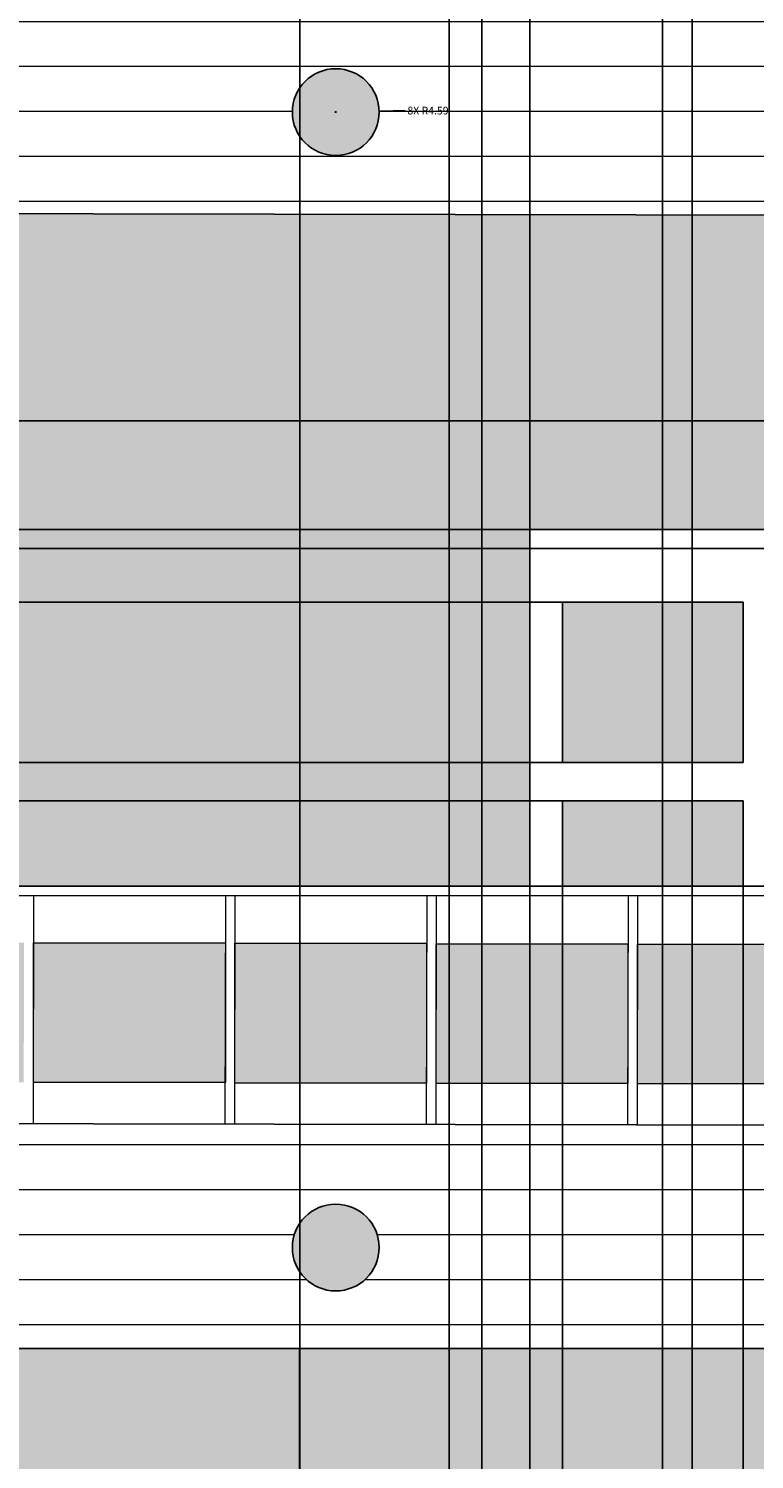
# Model space of a CAD drawing. Units: inches. Extents: x 36 to 594, y 79 to 831.
# Tile 9 of 30: x 188 to 265, y 294 to 446. Entities that reach past the tile are written whole.
import ezdxf

# ---------------------------------------------------------------- set-up
doc = ezdxf.new("R2010")
doc.units = ezdxf.units.IN
doc.header["$MEASUREMENT"] = 0
for name, color, linetype, lineweight in [('A-ANNO-DIMS', 2, 'Continuous', 18), ('A-ELEV', 7, 'Continuous', 25), ('A-ELEV-PATT', 8, 'Continuous', 13), ('A-GLAZ', 4, 'Continuous', 18)]:
    doc.layers.add(name, color=color, linetype=linetype, lineweight=lineweight)
doc.styles.get("Standard").update_dxf_attribs({"font": 'arial.ttf'})
doc.dimstyles.get("Standard").update_dxf_attribs({"dimtxt": 0.8125, "dimasz": 0.18, "dimexe": 0.18, "dimexo": 0.0625, "dimgap": 0.09, "dimtad": 0, "dimtih": 1, "dimtoh": 1, "dimdec": 4, "dimzin": 0, "dimdsep": 46, "dimlunit": 4, "dimtxsty": 'Standard', "dimcen": 0.09, "dimadec": 0, "dimazin": 0, "dimtfac": 1, "dimtdec": 4, "dimtofl": 0, "dimtmove": 0, "dimatfit": 3, "dimfxl": 1, "dimtolj": 1, "dimtzin": 0, "dimarcsym": 0})

# ---------------------------------------------------------------- blocks, each defined once
blk = doc.blocks.new('GLAZ-PANEL')
blk.add_lwpolyline([(0, 14.77), (20.28, 14.77), (20.28, 0), (0, 0)], close=True)
blk = doc.blocks.new('*D28')
at = {"layer": 'A-ANNO-DIMS', "color": 0, "lineweight": -2, "transparency": 16777216}
for p, q in [((269.3, 796.05), (37.49, 796.05)), ((37.67, 795.87), (37.67, 455.63)), ((37.67, 114.39), (37.67, 454.62)), ((94.8, 114.21), (37.49, 114.21))]:
    blk.add_line(p, q, dxfattribs=at)
at = {"layer": 'A-ANNO-DIMS', "color": 0, "transparency": 16777216}
for points in [[(37.64, 795.87), (37.7, 795.87), (37.67, 796.05)], [(37.64, 114.39), (37.7, 114.39), (37.67, 114.21)]]:
    blk.add_solid(points, dxfattribs=at)
at = {"layer": 'Defpoints', "color": 0, "transparency": 16777216}
for p in [(37.67, 796.05), (269.36, 796.05), (94.87, 114.21)]:
    blk.add_point(p, dxfattribs=at)
at = {"layer": 'A-ANNO-DIMS', "color": 0, "transparency": 16777216, "insert": (37.67, 455.13), "char_height": 0.812, "attachment_point": 5}
blk.add_mtext('\\A1;681.8', dxfattribs=at)
blk = doc.blocks.new('*D61')
at = {"layer": 'A-ANNO-DIMS', "color": 0, "lineweight": -2, "transparency": 16777216}
for p, q in [((156.41, 264.68), (156.41, 830.73)), ((156.59, 830.55), (185.26, 830.55)), ((216.85, 830.55), (188.18, 830.55)), ((217.03, 286.24), (217.03, 830.73))]:
    blk.add_line(p, q, dxfattribs=at)
at = {"layer": 'A-ANNO-DIMS', "color": 0, "transparency": 16777216}
for points in [[(156.59, 830.58), (156.59, 830.52), (156.41, 830.55)], [(216.85, 830.58), (216.85, 830.52), (217.03, 830.55)]]:
    blk.add_solid(points, dxfattribs=at)
at = {"layer": 'Defpoints', "color": 0, "transparency": 16777216}
for p in [(217.03, 830.55), (217.03, 286.18), (156.41, 264.62)]:
    blk.add_point(p, dxfattribs=at)
at = {"layer": 'A-ANNO-DIMS', "color": 0, "transparency": 16777216, "insert": (186.72, 830.55), "char_height": 0.812, "attachment_point": 5}
blk.add_mtext('\\A1;60.62', dxfattribs=at)
blk = doc.blocks.new('*D96')
at = {"layer": 'A-ANNO-DIMS', "color": 0, "lineweight": -2, "transparency": 16777216}
for p, q in [((236.29, 484.36), (236.29, 79.53)), ((232.82, 475.35), (232.82, 79.53)), ((233, 79.71), (233.41, 79.71)), ((236.11, 79.71), (235.7, 79.71))]:
    blk.add_line(p, q, dxfattribs=at)
at = {"layer": 'A-ANNO-DIMS', "color": 0, "transparency": 16777216}
for points in [[(233, 79.74), (233, 79.68), (232.82, 79.71)], [(236.11, 79.74), (236.11, 79.68), (236.29, 79.71)]]:
    blk.add_solid(points, dxfattribs=at)
at = {"layer": 'Defpoints', "color": 0, "transparency": 16777216}
for p in [(236.29, 484.42), (232.82, 475.41), (236.29, 79.71)]:
    blk.add_point(p, dxfattribs=at)
at = {"layer": 'A-ANNO-DIMS', "color": 0, "transparency": 16777216, "insert": (234.56, 79.71), "char_height": 0.812, "attachment_point": 5}
blk.add_mtext('\\A1;3.47', dxfattribs=at)
blk = doc.blocks.new('*D97')
at = {"layer": 'A-ANNO-DIMS', "color": 0, "lineweight": -2, "transparency": 16777216}
for p, q in [((236.29, 484.36), (236.29, 79.53)), ((255.36, 484.36), (255.36, 79.53)), ((236.47, 79.71), (244.09, 79.71)), ((255.18, 79.71), (247.56, 79.71))]:
    blk.add_line(p, q, dxfattribs=at)
at = {"layer": 'A-ANNO-DIMS', "color": 0, "transparency": 16777216}
for points in [[(236.47, 79.74), (236.47, 79.68), (236.29, 79.71)], [(255.18, 79.74), (255.18, 79.68), (255.36, 79.71)]]:
    blk.add_solid(points, dxfattribs=at)
at = {"layer": 'Defpoints', "color": 0, "transparency": 16777216}
for p in [(236.29, 484.42), (255.36, 484.42), (255.36, 79.71)]:
    blk.add_point(p, dxfattribs=at)
at = {"layer": 'A-ANNO-DIMS', "color": 0, "transparency": 16777216, "insert": (245.82, 79.71), "char_height": 0.812, "attachment_point": 5}
blk.add_mtext('\\A1;19.064', dxfattribs=at)
blk = doc.blocks.new('*D98')
at = {"layer": 'A-ANNO-DIMS', "color": 0, "lineweight": -2, "transparency": 16777216}
for p, q in [((255.36, 484.36), (255.36, 79.53)), ((258.51, 475.35), (258.51, 79.53)), ((255.54, 79.71), (255.78, 79.71)), ((258.33, 79.71), (258.08, 79.71))]:
    blk.add_line(p, q, dxfattribs=at)
at = {"layer": 'A-ANNO-DIMS', "color": 0, "transparency": 16777216}
for points in [[(255.54, 79.74), (255.54, 79.68), (255.36, 79.71)], [(258.33, 79.74), (258.33, 79.68), (258.51, 79.71)]]:
    blk.add_solid(points, dxfattribs=at)
at = {"layer": 'Defpoints', "color": 0, "transparency": 16777216}
for p in [(255.36, 484.42), (258.51, 475.41), (258.51, 79.71)]:
    blk.add_point(p, dxfattribs=at)
at = {"layer": 'A-ANNO-DIMS', "color": 0, "transparency": 16777216, "insert": (256.93, 79.71), "char_height": 0.812, "attachment_point": 5}
blk.add_mtext('\\A1;3.15', dxfattribs=at)
blk = doc.blocks.new('*D105')
at = {"layer": 'A-ANNO-DIMS', "color": 0, "lineweight": -2, "transparency": 16777216}
for p, q in [((241.36, 404.34), (241.36, 830.73)), ((241.54, 830.55), (252.42, 830.55)), ((266.86, 830.55), (255.98, 830.55)), ((267.04, 404.34), (267.04, 830.73))]:
    blk.add_line(p, q, dxfattribs=at)
at = {"layer": 'A-ANNO-DIMS', "color": 0, "transparency": 16777216}
for points in [[(241.54, 830.58), (241.54, 830.52), (241.36, 830.55)], [(266.86, 830.58), (266.86, 830.52), (267.04, 830.55)]]:
    blk.add_solid(points, dxfattribs=at)
at = {"layer": 'Defpoints', "color": 0, "transparency": 16777216}
for p in [(267.04, 830.55), (241.36, 404.27), (267.04, 404.27)]:
    blk.add_point(p, dxfattribs=at)
at = {"layer": 'A-ANNO-DIMS', "color": 0, "transparency": 16777216, "insert": (254.2, 830.55), "char_height": 0.812, "attachment_point": 5}
blk.add_mtext('\\A1;25.684', dxfattribs=at)
blk = doc.blocks.new('*D108')
at = {"layer": 'A-ANNO-DIMS', "color": 0, "lineweight": -2, "transparency": 16777216}
for p, q in [((244.82, 364.03), (244.82, 79.53)), ((241.36, 355.02), (241.36, 79.53)), ((241.54, 79.71), (241.95, 79.71)), ((244.64, 79.71), (244.24, 79.71))]:
    blk.add_line(p, q, dxfattribs=at)
at = {"layer": 'A-ANNO-DIMS', "color": 0, "transparency": 16777216}
for points in [[(241.54, 79.74), (241.54, 79.68), (241.36, 79.71)], [(244.64, 79.74), (244.64, 79.68), (244.82, 79.71)]]:
    blk.add_solid(points, dxfattribs=at)
at = {"layer": 'Defpoints', "color": 0, "transparency": 16777216}
for p in [(244.82, 364.09), (241.36, 355.08), (244.82, 79.71)]:
    blk.add_point(p, dxfattribs=at)
at = {"layer": 'A-ANNO-DIMS', "color": 0, "transparency": 16777216, "insert": (243.09, 79.71), "char_height": 0.812, "attachment_point": 5}
blk.add_mtext('\\A1;3.47', dxfattribs=at)
blk = doc.blocks.new('*D109')
at = {"layer": 'A-ANNO-DIMS', "color": 0, "lineweight": -2, "transparency": 16777216}
for p, q in [((244.82, 364.03), (244.82, 79.53)), ((263.89, 364.03), (263.89, 79.53)), ((245, 79.71), (252.62, 79.71)), ((263.71, 79.71), (256.09, 79.71))]:
    blk.add_line(p, q, dxfattribs=at)
at = {"layer": 'A-ANNO-DIMS', "color": 0, "transparency": 16777216}
for points in [[(245, 79.74), (245, 79.68), (244.82, 79.71)], [(263.71, 79.74), (263.71, 79.68), (263.89, 79.71)]]:
    blk.add_solid(points, dxfattribs=at)
at = {"layer": 'Defpoints', "color": 0, "transparency": 16777216}
for p in [(244.82, 364.09), (263.89, 364.09), (263.89, 79.71)]:
    blk.add_point(p, dxfattribs=at)
at = {"layer": 'A-ANNO-DIMS', "color": 0, "transparency": 16777216, "insert": (254.36, 79.71), "char_height": 0.812, "attachment_point": 5}
blk.add_mtext('\\A1;19.064', dxfattribs=at)
blk = doc.blocks.new('*D110')
at = {"layer": 'A-ANNO-DIMS', "color": 0, "lineweight": -2, "transparency": 16777216}
for p, q in [((263.89, 364.03), (263.89, 79.53)), ((267.04, 355.02), (267.04, 79.53)), ((264.07, 79.71), (264.32, 79.71)), ((266.86, 79.71), (266.61, 79.71))]:
    blk.add_line(p, q, dxfattribs=at)
at = {"layer": 'A-ANNO-DIMS', "color": 0, "transparency": 16777216}
for points in [[(264.07, 79.74), (264.07, 79.68), (263.89, 79.71)], [(266.86, 79.74), (266.86, 79.68), (267.04, 79.71)]]:
    blk.add_solid(points, dxfattribs=at)
at = {"layer": 'Defpoints', "color": 0, "transparency": 16777216}
for p in [(263.89, 364.09), (267.04, 355.08), (267.04, 79.71)]:
    blk.add_point(p, dxfattribs=at)
at = {"layer": 'A-ANNO-DIMS', "color": 0, "transparency": 16777216, "insert": (265.46, 79.71), "char_height": 0.812, "attachment_point": 5}
blk.add_mtext('\\A1;3.15', dxfattribs=at)
blk = doc.blocks.new('*D111')
at = {"layer": 'A-ANNO-DIMS', "color": 0, "lineweight": -2, "transparency": 16777216}
for p, q in [((244.76, 364.09), (37.49, 364.09)), ((37.67, 363.91), (37.67, 360.09)), ((37.67, 355.26), (37.67, 359.08)), ((241.29, 355.08), (37.49, 355.08))]:
    blk.add_line(p, q, dxfattribs=at)
at = {"layer": 'A-ANNO-DIMS', "color": 0, "transparency": 16777216}
for points in [[(37.64, 363.91), (37.7, 363.91), (37.67, 364.09)], [(37.64, 355.26), (37.7, 355.26), (37.67, 355.08)]]:
    blk.add_solid(points, dxfattribs=at)
at = {"layer": 'Defpoints', "color": 0, "transparency": 16777216}
for p in [(37.67, 364.09), (244.82, 364.09), (241.36, 355.08)]:
    blk.add_point(p, dxfattribs=at)
at = {"layer": 'A-ANNO-DIMS', "color": 0, "transparency": 16777216, "insert": (37.67, 359.59), "char_height": 0.812, "attachment_point": 5}
blk.add_mtext('\\A1;9.005', dxfattribs=at)
blk = doc.blocks.new('*D112')
at = {"layer": 'A-ANNO-DIMS', "color": 0, "lineweight": -2, "transparency": 16777216}
for p, q in [((244.76, 368.16), (37.49, 368.16)), ((37.67, 367.98), (37.67, 366.63)), ((37.67, 364.27), (37.67, 365.62)), ((244.76, 364.09), (37.49, 364.09))]:
    blk.add_line(p, q, dxfattribs=at)
at = {"layer": 'A-ANNO-DIMS', "color": 0, "transparency": 16777216}
for points in [[(37.64, 367.98), (37.7, 367.98), (37.67, 368.16)], [(37.64, 364.27), (37.7, 364.27), (37.67, 364.09)]]:
    blk.add_solid(points, dxfattribs=at)
at = {"layer": 'Defpoints', "color": 0, "transparency": 16777216}
for p in [(37.67, 368.16), (244.82, 368.16), (244.82, 364.09)]:
    blk.add_point(p, dxfattribs=at)
at = {"layer": 'A-ANNO-DIMS', "color": 0, "transparency": 16777216, "insert": (37.67, 366.13), "char_height": 0.812, "attachment_point": 5}
blk.add_mtext('\\A1;4.074', dxfattribs=at)
blk = doc.blocks.new('*D113')
at = {"layer": 'A-ANNO-DIMS', "color": 0, "lineweight": -2, "transparency": 16777216}
for p, q in [((244.76, 385.12), (37.49, 385.12)), ((37.67, 384.94), (37.67, 377.15)), ((37.67, 368.34), (37.67, 376.14)), ((244.76, 368.16), (37.49, 368.16))]:
    blk.add_line(p, q, dxfattribs=at)
at = {"layer": 'A-ANNO-DIMS', "color": 0, "transparency": 16777216}
for points in [[(37.64, 384.94), (37.7, 384.94), (37.67, 385.12)], [(37.64, 368.34), (37.7, 368.34), (37.67, 368.16)]]:
    blk.add_solid(points, dxfattribs=at)
at = {"layer": 'Defpoints', "color": 0, "transparency": 16777216}
for p in [(37.67, 385.12), (244.82, 385.12), (244.82, 368.16)]:
    blk.add_point(p, dxfattribs=at)
at = {"layer": 'A-ANNO-DIMS', "color": 0, "transparency": 16777216, "insert": (37.67, 376.64), "char_height": 0.812, "attachment_point": 5}
blk.add_mtext('\\A1;16.957', dxfattribs=at)
blk = doc.blocks.new('*D114')
at = {"layer": 'A-ANNO-DIMS', "color": 0, "lineweight": -2, "transparency": 16777216}
for p, q in [((241.29, 390.79), (37.49, 390.79)), ((37.67, 390.61), (37.67, 388.46)), ((37.67, 385.3), (37.67, 387.45)), ((244.76, 385.12), (37.49, 385.12))]:
    blk.add_line(p, q, dxfattribs=at)
at = {"layer": 'A-ANNO-DIMS', "color": 0, "transparency": 16777216}
for points in [[(37.64, 390.61), (37.7, 390.61), (37.67, 390.79)], [(37.64, 385.3), (37.7, 385.3), (37.67, 385.12)]]:
    blk.add_solid(points, dxfattribs=at)
at = {"layer": 'Defpoints', "color": 0, "transparency": 16777216}
for p in [(37.67, 390.79), (241.36, 390.79), (244.82, 385.12)]:
    blk.add_point(p, dxfattribs=at)
at = {"layer": 'A-ANNO-DIMS', "color": 0, "transparency": 16777216, "insert": (37.67, 387.96), "char_height": 0.812, "attachment_point": 5}
blk.add_mtext('\\A1;5.672', dxfattribs=at)
blk = doc.blocks.new('*D115')
at = {"layer": 'A-ANNO-DIMS', "color": 0, "lineweight": -2, "transparency": 16777216}
for p, q in [((241.29, 392.79), (37.49, 392.79)), ((37.67, 392.61), (37.67, 392.29)), ((241.29, 390.79), (37.49, 390.79)), ((37.67, 390.97), (37.67, 391.29))]:
    blk.add_line(p, q, dxfattribs=at)
at = {"layer": 'A-ANNO-DIMS', "color": 0, "transparency": 16777216}
for points in [[(37.64, 392.61), (37.7, 392.61), (37.67, 392.79)], [(37.64, 390.97), (37.7, 390.97), (37.67, 390.79)]]:
    blk.add_solid(points, dxfattribs=at)
at = {"layer": 'Defpoints', "color": 0, "transparency": 16777216}
for p in [(37.67, 392.79), (241.36, 392.79), (241.36, 390.79)]:
    blk.add_point(p, dxfattribs=at)
at = {"layer": 'A-ANNO-DIMS', "color": 0, "transparency": 16777216, "insert": (37.67, 391.79), "char_height": 0.812, "attachment_point": 5}
blk.add_mtext('\\A1;2', dxfattribs=at)
blk = doc.blocks.new('*D116')
at = {"layer": 'A-ANNO-DIMS', "color": 0, "lineweight": -2, "transparency": 16777216}
for p, q in [((241.29, 404.27), (37.49, 404.27)), ((37.67, 404.09), (37.67, 399.04)), ((37.67, 392.97), (37.67, 398.03)), ((241.29, 392.79), (37.49, 392.79))]:
    blk.add_line(p, q, dxfattribs=at)
at = {"layer": 'A-ANNO-DIMS', "color": 0, "transparency": 16777216}
for points in [[(37.64, 404.09), (37.7, 404.09), (37.67, 404.27)], [(37.64, 392.97), (37.7, 392.97), (37.67, 392.79)]]:
    blk.add_solid(points, dxfattribs=at)
at = {"layer": 'Defpoints', "color": 0, "transparency": 16777216}
for p in [(37.67, 404.27), (241.36, 404.27), (241.36, 392.79)]:
    blk.add_point(p, dxfattribs=at)
at = {"layer": 'A-ANNO-DIMS', "color": 0, "transparency": 16777216, "insert": (37.67, 398.53), "char_height": 0.812, "attachment_point": 5}
blk.add_mtext('\\A1;11.481', dxfattribs=at)
blk = doc.blocks.new('*D130')
at = {"layer": 'A-ANNO-DIMS', "color": 0, "lineweight": -2, "transparency": 16777216}
for p, q in [((220.75, 436.91), (220.93, 436.91)), ((220.84, 436.82), (220.84, 437)), ((228.18, 437.07), (225.61, 437.01))]:
    blk.add_line(p, q, dxfattribs=at)
at = {"layer": 'A-ANNO-DIMS', "color": 0, "transparency": 16777216}
blk.add_solid([(225.61, 437.04), (225.61, 436.98), (225.43, 437.01)], dxfattribs=at)
at = {"layer": 'Defpoints', "color": 0, "transparency": 16777216}
for p in [(220.84, 436.91), (225.43, 437.01)]:
    blk.add_point(p, dxfattribs=at)
at = {"layer": 'A-ANNO-DIMS', "color": 0, "transparency": 16777216, "insert": (230.59, 437.07), "char_height": 0.8125, "attachment_point": 5}
blk.add_mtext('\\A1;8X R4.59', dxfattribs=at)

msp = doc.modelspace()

# ---------------------------------------------------------------- hatches: boundary and pattern name
at = {"layer": 'A-ELEV-PATT'}
h = msp.add_hatch(color=256, dxfattribs=at)
h.dxf.hatch_style = 1
h.paths.add_polyline_path([(398.0873, 796.0465), (269.3592, 796.0465), (269.3592, 770.1455), (397.8159, 770.1455)])
h.paths.add_polyline_path([(397.7518, 764.0341), (269.3592, 764.0341), (269.3592, 630.0394), (341.8367, 630.0394), (341.8367, 720.595), (335.0881, 728.3699), (329.982, 735.3373), (345.3661, 727.7743), (397.1052, 702.3389)])
h.paths.add_polyline_path([(341.8367, 594.2124), (201.4189, 594.2124), (201.4189, 475.4136), (232.8216, 475.4136), (232.8216, 524.6037), (341.8367, 524.6037)])
h.paths.add_polyline_path([(177.525, 594.2124), (118.7598, 594.2124), (118.7598, 450.2124), (177.525, 450.2124)])
h.paths.add_polyline_path([(424.4958, 594.2124), (365.7306, 594.2124), (365.7306, 450.2124), (424.4958, 450.2124)])
h.paths.add_polyline_path([(241.3553, 404.2737), (355.8569, 404.2737), (355.8569, 355.0836), (424.5492, 355.0836), (424.5492, 425.7333), (118.7598, 426.2844), (118.7598, 355.0836), (241.3553, 355.0836)])
h.paths.add_polyline_path([(448.3898, 306.2124), (217.0273, 306.2124), (217.0273, 142.2124), (254.0293, 142.2124), (254.0293, 150.9347), (254.0293, 286.1802), (401.5491, 286.1802), (401.5491, 150.9347), (401.5491, 142.2124), (448.3898, 142.2124)])
h.paths.add_polyline_path([(448.3898, 142.2124), (401.5491, 142.2124), (217.0273, 142.2124), (217.0273, 114.2124), (448.3898, 114.2124)])
h.paths.add_polyline_path([(217.0273, 306.2124), (174.7353, 306.2124), (94.8658, 306.2124), (94.8658, 162.2124), (103.3368, 162.2124), (103.3368, 264.6224), (103.3368, 286.1802), (217.0273, 286.1802)])
h = msp.add_hatch(color=256, dxfattribs=at)
h.dxf.hatch_style = 1
h.set_gradient(color1=(0, 255, 255), color2=(16, 86, 137))
h.paths.add_polyline_path([(341.8367, 524.6037), (260.5056, 524.6037), (260.5056, 513.1224), (341.8367, 513.1224)])
h.paths.add_polyline_path([(341.8367, 511.1224), (260.5056, 511.1224), (260.5056, 475.4136), (341.8367, 475.4136)])
h.paths.add_polyline_path([(258.5056, 524.6037), (232.8216, 524.6037), (232.8216, 513.1224), (258.5056, 513.1224)])
h.paths.add_polyline_path([(355.8569, 404.2737), (269.0393, 404.2737), (269.0393, 392.7924), (355.8569, 392.7924)])
h.paths.add_polyline_path([(267.0393, 404.2737), (241.3553, 404.2737), (241.3553, 392.7924), (267.0393, 392.7924)])
h.paths.add_polyline_path([(355.8569, 390.7924), (269.0393, 390.7924), (269.0393, 355.0836), (355.8569, 355.0836)])
h.paths.add_polyline_path([(399.5491, 284.1802), (256.0293, 284.1802), (256.0293, 271.378), (399.5491, 271.378)])
h.paths.add_polyline_path([(317.3533, 259.1243), (262.3169, 259.1243), (262.3169, 200.6645), (317.3533, 200.6645)])
h.paths.add_polyline_path([(390.386, 259.1243), (335.3496, 259.1243), (335.3496, 200.6645), (390.386, 200.6645)])
h.paths.add_polyline_path([(390.386, 190.7697), (335.3496, 190.7697), (335.3496, 162.9881), (390.386, 162.9881)])
h.paths.add_polyline_path([(317.3533, 190.7697), (262.3169, 190.7697), (262.3169, 162.9881), (317.3533, 162.9881)])
h.paths.add_polyline_path([(215.0273, 262.6224), (158.4069, 262.6224), (158.4069, 181.4195), (215.0273, 181.4195)])
h.paths.add_polyline_path([(215.0273, 284.1802), (105.3368, 284.1802), (105.3368, 266.6224), (215.0273, 266.6224)])
h = msp.add_hatch(dxfattribs=at)
h.set_pattern_fill('ANSI33', color=256, scale=6.3, angle=135)
h.paths.add_polyline_path([(255.3555, 505.4499), (236.2911, 505.4499), (236.2911, 488.4928), (255.3555, 488.4928)])
h.paths.add_polyline_path([(255.3555, 484.4187), (236.2911, 484.4187), (236.2911, 475.4136), (255.3555, 475.4136)])
h.paths.add_polyline_path([(263.8892, 385.1199), (244.8248, 385.1199), (244.8248, 368.1628), (263.8892, 368.1628)])
h.paths.add_polyline_path([(263.8892, 364.0887), (244.8248, 364.0887), (244.8248, 355.0836), (263.8892, 355.0836)])
h.paths.add_polyline_path([(148.0383, 248.8663), (113.6593, 248.8663), (113.6593, 214.2237), (148.0383, 214.2237)])
h.paths.add_polyline_path([(148.0383, 203.057), (113.6593, 203.057), (113.6593, 170.5978), (148.0383, 170.5978)])
h = msp.add_hatch(color=256, dxfattribs=at)
h.dxf.hatch_style = 1
h.set_gradient(color1=(192, 192, 192), color2=(0, 0, 0))
h.paths.add_polyline_path([(243.19, 469.3251), (222.9132, 469.3251), (222.9132, 454.5571), (243.1634, 454.5571)])
h.paths.add_polyline_path([(264.4667, 469.2868), (244.1899, 469.2868), (244.1899, 454.5188), (264.4401, 454.5188)])
h.paths.add_polyline_path([(285.7435, 469.2484), (265.4667, 469.2484), (265.4667, 454.4804), (285.7168, 454.4804)])
h.paths.add_polyline_path([(307.0202, 469.2101), (286.7434, 469.2101), (286.7434, 454.4421), (306.9936, 454.4421)])
h.paths.add_polyline_path([(328.2969, 469.1717), (308.0201, 469.1717), (308.0201, 454.4037), (328.2703, 454.4037)])
h.paths.add_polyline_path([(341.8367, 469.1334), (329.2969, 469.1334), (329.2969, 454.3654), (341.8367, 454.3654)])
h.paths.add_polyline_path([(221.9133, 469.3635), (201.6365, 469.3635), (201.6365, 454.5955), (221.8866, 454.5955)])
h.paths.add_polyline_path([(145.3401, 349.1868), (125.0633, 349.1868), (125.0633, 334.4189), (145.3134, 334.4189)])
h.paths.add_polyline_path([(166.6168, 349.1485), (146.34, 349.1485), (146.34, 334.3805), (166.5902, 334.3805)])
h.paths.add_polyline_path([(187.8935, 349.1101), (167.6167, 349.1101), (167.6167, 334.3422), (187.8669, 334.3422)])
h.paths.add_polyline_path([(209.1703, 349.0718), (188.8935, 349.0718), (188.8935, 334.3038), (209.1436, 334.3038)])
h.paths.add_polyline_path([(230.447, 349.0335), (210.1702, 349.0335), (210.1702, 334.2655), (230.4204, 334.2655)])
h.paths.add_polyline_path([(251.7237, 348.9951), (231.4469, 348.9951), (231.4469, 334.2271), (251.6971, 334.2271)])
h.paths.add_polyline_path([(273.0005, 348.9568), (252.7236, 348.9568), (252.7236, 334.1888), (272.9738, 334.1888)])
h.paths.add_polyline_path([(294.2772, 348.9184), (274.0004, 348.9184), (274.0004, 334.1504), (294.2506, 334.1504)])
h.paths.add_polyline_path([(315.5539, 348.8801), (295.2771, 348.8801), (295.2771, 334.1121), (315.5273, 334.1121)])
h.paths.add_polyline_path([(336.8306, 348.8417), (316.5538, 348.8417), (316.5538, 334.0737), (336.804, 334.0737)])
h.paths.add_polyline_path([(358.1074, 348.8034), (337.8306, 348.8034), (337.8306, 334.0354), (358.0808, 334.0354)])
h.paths.add_polyline_path([(379.3841, 348.765), (359.1073, 348.765), (359.1073, 333.997), (379.3575, 333.997)])
h.paths.add_polyline_path([(400.6608, 348.7267), (380.384, 348.7267), (380.384, 333.9587), (400.6342, 333.9587)])
h.paths.add_polyline_path([(421.9376, 348.6883), (401.6608, 348.6883), (401.6608, 333.9204), (421.911, 333.9204)])
h.paths.add_polyline_path([(103.3368, 162.2124), (94.8658, 162.2124), (94.8658, 150.2124), (94.8658, 114.2124), (103.3368, 114.2124)])
h.paths.add_polyline_path([(217.0273, 132.2124), (103.3368, 132.2124), (103.3368, 122.2124), (217.0273, 122.2124)])
h.paths.add_polyline_path([(217.0273, 122.2124), (103.3368, 122.2124), (103.3368, 114.2124), (217.0273, 114.2124)])
h.paths.add_polyline_path([(217.0273, 142.2124), (174.7353, 142.2124), (103.3368, 142.2124), (103.3368, 132.2124), (217.0273, 132.2124)])
h.paths.add_polyline_path([(217.0273, 152.2124), (103.3368, 152.2124), (103.3368, 142.2124), (174.7353, 142.2124), (217.0273, 142.2124)])
h.paths.add_polyline_path([(217.0273, 162.2124), (103.3368, 162.2124), (103.3368, 152.2124), (217.0273, 152.2124)])
h = msp.add_hatch(dxfattribs=at)
h.set_pattern_fill('ANSI31', color=256, scale=38, angle=135)
h.paths.add_polyline_path([(448.3898, 450.2124), (94.8658, 450.2124), (94.8658, 306.2124), (174.7353, 306.2124), (448.3898, 306.2124), (448.3898, 367.5118)])
h.paths.add_polyline_path([(424.5492, 425.7333), (424.5492, 329.5325), (118.7598, 330.0836), (118.7598, 354.0836), (118.7598, 426.2844)], flags=16)
h.paths.add_polyline_path([(355.8569, 404.2737), (355.8569, 355.0836), (241.3553, 355.0836), (241.3553, 404.2737)], flags=0)
h.paths.add_polyline_path([(269.0393, 390.7924), (269.0393, 355.0836), (244.8248, 355.0836), (244.8248, 364.0887), (263.8892, 364.0887), (263.8892, 355.0836), (267.0393, 355.0836), (267.0393, 390.7924)], flags=0)
h.paths.add_polyline_path([(303.9765, 436.9126, -1), (313.1496, 436.9126, -1)], flags=16)
h.paths.add_polyline_path([(421.9473, 354.0836), (421.9376, 348.6883), (421.9376, 333.9204), (401.6342, 333.9204), (401.6705, 354.0836), (400.6705, 354.0836), (400.6608, 348.7267), (400.6608, 333.9587), (380.3574, 333.9587), (380.3937, 354.0836), (379.3937, 354.0836), (379.3841, 348.765), (379.3841, 333.997), (359.0807, 333.997), (359.1169, 354.0836), (358.1169, 354.0836), (358.1074, 348.8034), (358.1074, 334.0354), (337.804, 334.0354), (337.8401, 354.0836), (336.8401, 354.0836), (336.8306, 348.8417), (336.8306, 334.0737), (316.5272, 334.0737), (316.5633, 354.0836), (315.5633, 354.0836), (315.5539, 348.8801), (315.5539, 334.1121), (295.2505, 334.1121), (295.2865, 354.0836), (294.2865, 354.0836), (294.2772, 348.9184), (294.2772, 334.1504), (273.9738, 334.1504), (274.0097, 354.0836), (273.0097, 354.0836), (273.0005, 348.9568), (273.0005, 334.1888), (252.697, 334.1888), (252.7329, 354.0836), (251.7329, 354.0836), (251.7237, 348.9951), (251.7237, 334.2271), (231.4203, 334.2271), (231.4561, 354.0836), (230.4561, 354.0836), (230.447, 349.0335), (230.447, 334.2655), (210.1436, 334.2655), (210.1793, 354.0836), (209.1793, 354.0836), (209.1703, 349.0718), (209.1703, 334.3038), (188.8668, 334.3038), (188.9025, 354.0836), (187.9025, 354.0836), (187.8935, 349.1101), (187.8935, 334.3422), (167.5901, 334.3422), (167.6257, 354.0836), (166.6257, 354.0836), (166.6168, 349.1485), (166.6168, 334.3805), (146.3134, 334.3805), (146.3489, 354.0836), (145.3489, 354.0836), (145.3401, 349.1868), (145.3401, 334.4189), (125.0366, 334.4189), (125.0721, 354.0836)], flags=0)
h.paths.add_polyline_path([(266.285, 436.9126, -1), (275.458, 436.9126, -1)], flags=16)
h.paths.add_polyline_path([(367.0204, 316.8739, -1), (357.8474, 316.8739, -1)], flags=16)
h.paths.add_polyline_path([(347.6933, 316.8739, -1), (338.5202, 316.8739, -1)], flags=16)
h.paths.add_polyline_path([(329.574, 316.8739, -1), (320.401, 316.8739, -1)], flags=16)
h.paths.add_polyline_path([(263.8892, 385.1199), (263.8892, 368.1628), (244.8248, 368.1628), (244.8248, 385.1199)], flags=0)
h.paths.add_polyline_path([(216.2543, 436.9126, -1), (225.4274, 436.9126, -1)], flags=16)
h.paths.add_polyline_path([(275.458, 316.8739, -1), (266.285, 316.8739, -1)], flags=16)
h.paths.add_polyline_path([(225.4274, 316.8739, -1), (216.2543, 316.8739, -1)], flags=16)
h = msp.add_hatch(color=256, dxfattribs=at)
h.dxf.hatch_style = 1
h.paths.add_polyline_path([(313.1496, 436.9126, 1), (303.9765, 436.9126, 1)])
h.paths.add_polyline_path([(266.285, 436.9126, 1), (275.458, 436.9126, 1)])
h.paths.add_polyline_path([(225.4274, 436.9126, 1), (216.2543, 436.9126, 1)])
h.paths.add_polyline_path([(329.574, 316.8739, 1), (320.401, 316.8739, 1)])
h.paths.add_polyline_path([(347.6933, 316.8739, 1), (338.5202, 316.8739, 1)])
h.paths.add_polyline_path([(357.8474, 316.8739, 1), (367.0204, 316.8739, 1)])
h.paths.add_polyline_path([(275.458, 316.8739, 1), (266.285, 316.8739, 1)])
h.paths.add_polyline_path([(216.2543, 316.8739, 1), (225.4274, 316.8739, 1)])

# ---------------------------------------------------------------- linework, layer by layer
at = {"layer": 'A-ELEV'}
for p, q in [((241.3553, 392.7924), (355.8569, 392.7924)), ((241.3553, 390.7924), (355.8569, 390.7924)), ((174.7353, 306.2124), (448.3898, 306.2124)), ((217.0273, 114.2124), (217.0273, 306.2124))]:
    msp.add_line(p, q, dxfattribs=at)
for points in [[(118.7598, 426.2844), (424.5492, 425.7333), (424.5492, 329.5325), (118.7598, 330.0836)], [(241.3553, 404.2737), (355.8569, 404.2737), (355.8569, 355.0836), (241.3553, 355.0836)], [(244.8248, 385.1199), (263.8892, 385.1199), (263.8892, 368.1628), (244.8248, 368.1628)], [(244.8248, 364.0887), (263.8892, 364.0887), (263.8892, 355.0836), (244.8248, 355.0836)]]:
    msp.add_lwpolyline(points, close=True, dxfattribs=at)
for centre in [(220.8408, 436.9126), (220.8408, 316.8739)]:
    msp.add_circle(centre, 4.5865, dxfattribs=at)
at = {"layer": 'A-GLAZ'}
for p, q in [((118.7598, 355.0836), (424.5492, 355.0836)), ((118.7598, 354.0836), (424.5492, 354.0836)), ((188.9025, 354.0836), (188.8591, 329.9956)), ((209.1793, 354.0836), (209.1358, 329.9591)), ((210.1793, 354.0836), (210.1358, 329.9572)), ((230.4561, 354.0836), (230.4125, 329.9207)), ((231.4561, 354.0836), (231.4125, 329.9189)), ((251.7329, 354.0836), (251.6893, 329.8824)), ((252.7329, 354.0836), (252.6893, 329.8806))]:
    msp.add_line(p, q, dxfattribs=at)

# ---------------------------------------------------------------- block references
for p in [(188.8932, 334.304), (210.1699, 334.2656), (231.4467, 334.2273), (252.7234, 334.1889)]:
    msp.add_blockref('GLAZ-PANEL', p, dxfattribs=at)

# ---------------------------------------------------------------- dimensions: what is measured, and where the dimension line sits
at = {"layer": 'A-ANNO-DIMS'}
for base, p1, p2, override, picture, middle in [((217.0273, 830.5465), (156.4069, 264.6224), (217.0273, 286.1802), {"dimdec": 2, "dimlfac": 1, "dimrnd": 0, "dimzin": 0, "dimdsep": 46, "dimlunit": 2}, '*D61', (186.7171, 830.5465)), ((267.0393, 830.5465), (241.3553, 404.2737), (267.0393, 404.2737), {"dimdec": 3, "dimlfac": 1, "dimrnd": 0, "dimzin": 0, "dimdsep": 46, "dimlunit": 2}, '*D105', (254.1973, 830.5465)), ((236.2911, 79.7124), (232.8216, 475.4136), (236.2911, 484.4187), {"dimdec": 2, "dimlfac": 1, "dimrnd": 0, "dimzin": 0, "dimdsep": 46, "dimlunit": 2}, '*D96', (234.5563, 79.7124)), ((255.3555, 79.7124), (236.2911, 484.4187), (255.3555, 484.4187), {"dimdec": 3, "dimlfac": 1, "dimrnd": 0, "dimzin": 0, "dimdsep": 46, "dimlunit": 2}, '*D97', (245.8233, 79.7124)), ((258.5056, 79.7124), (255.3555, 484.4187), (258.5056, 475.4136), {"dimdec": 2, "dimlfac": 1, "dimrnd": 0, "dimzin": 0, "dimdsep": 46, "dimlunit": 2}, '*D98', (256.9305, 79.7124)), ((244.8248, 79.7124), (241.3553, 355.0836), (244.8248, 364.0887), {"dimdec": 2, "dimlfac": 1, "dimrnd": 0, "dimzin": 0, "dimdsep": 46, "dimlunit": 2}, '*D108', (243.09, 79.7124)), ((263.8892, 79.7124), (244.8248, 364.0887), (263.8892, 364.0887), {"dimdec": 3, "dimlfac": 1, "dimrnd": 0, "dimzin": 0, "dimdsep": 46, "dimlunit": 2}, '*D109', (254.357, 79.7124)), ((267.0393, 79.7124), (263.8892, 364.0887), (267.0393, 355.0836), {"dimdec": 2, "dimlfac": 1, "dimrnd": 0, "dimzin": 0, "dimdsep": 46, "dimlunit": 2}, '*D110', (265.4643, 79.7124))]:
    dim = msp.add_linear_dim(base=base, p1=p1, p2=p2, dimstyle='Standard', override=override, dxfattribs=at)
    dim.commit()
    dim.dimension.update_dxf_attribs({"geometry": picture, "text_midpoint": middle})
for base, p1, p2, override, picture, middle in [((37.6733, 796.0465), (94.8658, 114.2124), (269.3592, 796.0465), {"dimdec": 1, "dimlfac": 1, "dimrnd": 0, "dimzin": 0, "dimdsep": 46, "dimlunit": 2}, '*D28', (37.6733, 455.1294)), ((37.6733, 404.2737), (241.3553, 392.7924), (241.3553, 404.2737), {"dimdec": 3, "dimlfac": 1, "dimrnd": 0, "dimzin": 0, "dimdsep": 46, "dimlunit": 2}, '*D116', (37.6733, 398.533)), ((37.6733, 392.7924), (241.3553, 390.7924), (241.3553, 392.7924), {"dimdec": 0, "dimlfac": 1, "dimrnd": 0, "dimzin": 0, "dimdsep": 46, "dimlunit": 2}, '*D115', (37.6733, 391.7924)), ((37.67335, 390.79236), (244.82478, 385.11988), (241.3553, 390.79236), {"dimdec": 3, "dimlfac": 1, "dimrnd": 0, "dimzin": 0, "dimdsep": 46, "dimlunit": 2}, '*D114', (37.67335, 387.95612)), ((37.6733, 385.1199), (244.8248, 368.1628), (244.8248, 385.1199), {"dimdec": 3, "dimlfac": 1, "dimrnd": 0, "dimzin": 0, "dimdsep": 46, "dimlunit": 2}, '*D113', (37.6733, 376.6414)), ((37.6733, 368.1628), (244.8248, 364.0887), (244.8248, 368.1628), {"dimdec": 3, "dimlfac": 1, "dimrnd": 0, "dimzin": 0, "dimdsep": 46, "dimlunit": 2}, '*D112', (37.6733, 366.1258)), ((37.6733, 364.0887), (241.3553, 355.0836), (244.8248, 364.0887), {"dimdec": 3, "dimlfac": 1, "dimrnd": 0, "dimzin": 0, "dimdsep": 46, "dimlunit": 2}, '*D111', (37.6733, 359.5862))]:
    dim = msp.add_linear_dim(base=base, p1=p1, p2=p2, angle=90, dimstyle='Standard', override=override, dxfattribs=at)
    dim.commit()
    dim.dimension.update_dxf_attribs({"geometry": picture, "text_midpoint": middle})
dim = msp.add_radius_dim(center=(220.8408, 436.9126), mpoint=(225.4264, 437.009), text='8X <>', dimstyle='Standard', override={"dimdec": 2, "dimlfac": 1, "dimrnd": 0, "dimzin": 0, "dimdsep": 46, "dimlunit": 2}, dxfattribs=at)
dim.commit()
dim.dimension.update_dxf_attribs({"geometry": '*D130', "text_midpoint": (228.1777, 437.0667), "dimtype": 164})

doc.saveas('drawing.dxf')
